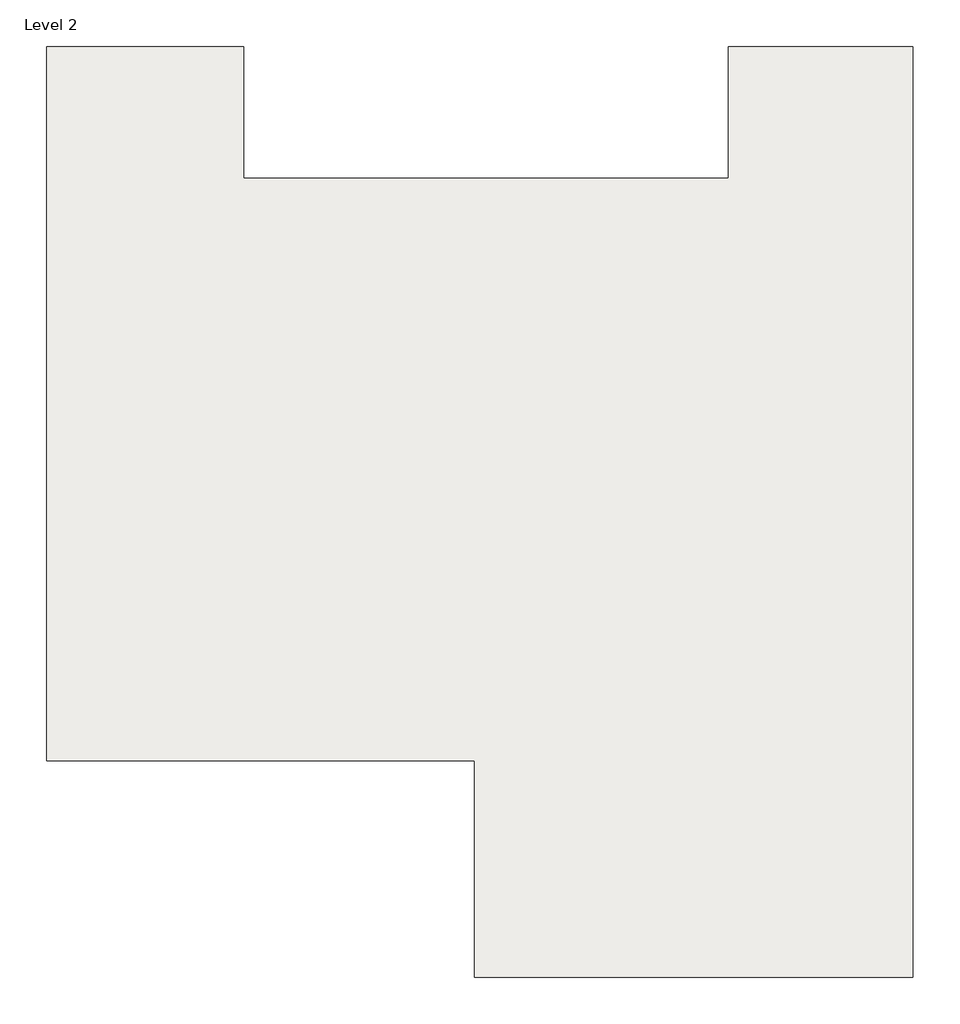
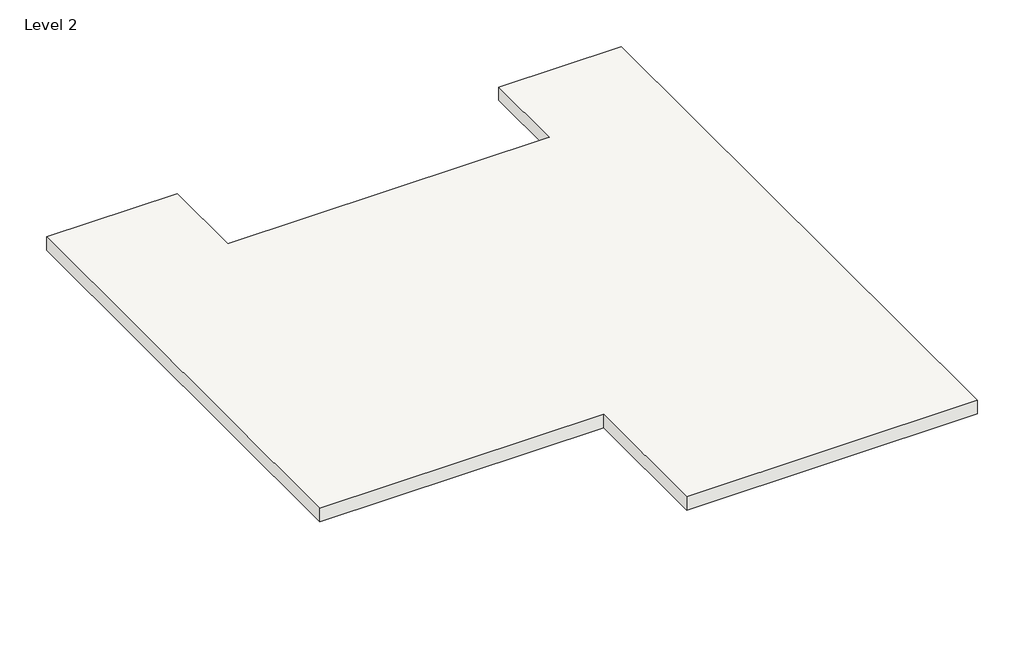
# One storey: 1 roof.
"""IFC4 building model written with IfcOpenShell, lengths in millimetres."""

from ifc_helpers import new_model, si_unit, frame, origin, place, context, project, spatial, polyline, outline, extrude, element, save

model = new_model("IFC4")

# Units and contexts
model_context = context("Model", 3, world=origin())
ifc_project = project(units=[si_unit("LENGTHUNIT", "METRE", prefix="MILLI")], contexts=[model_context])

# Site, building, storey
site = spatial("IfcSite", under=ifc_project)
building = spatial("IfcBuilding", under=site)
storey = spatial("IfcBuildingStorey", under=building, Name="Level 2", Elevation=3048.0)

# Roof
placement = place(None, origin())
element("IfcRoof", 1, ObjectType="Generic - 12\"", at=placement, inside=storey, context=model_context, shape_type="SweptSolid", body=[
    extrude(outline(polyline([(-392.7238552, 14768.0234128), (-392.7238552, 1547.3234128), (-392.7238552, 1458.4234128), (-6666.5238552, 1458.4234128), (-6666.5238552, 4557.2234128), (-12787.9238552, 4557.2234128), (-12787.9238552, 14768.0234128), (-9968.5238552, 14768.0234128), (-9968.5238552, 12888.4234128), (-3034.3238552, 12888.4234128), (-3034.3238552, 14768.0234128), (-392.7238552, 14768.0234128)])), frame((0.0, 0.0, 3048.0), z_axis=(0.0, 0.0, 1.0), x_axis=(1.0, 0.0, 0.0)), (0.0, 0.0, 1.0), 304.8),
])

save(model, "model.ifc")

# Revit data of these elements
# Type "Generic - 12\""
#   Assembly Code = "B1020"
#   Layers, outside or top first: 1' - 0" "Brick, Soldier Course" (function 1)
# Element 1 (IfcRoof, "Generic - 12\"")
#   built-in parameter 1001705 = 11 (stored number, unit not read)
#   built-in parameter 1001710 = 33615
#   Phase Created = New Construction
#   Materials on its faces: "Brick, Soldier Course"
# Materials
#   "Brick, Soldier Course": class "Masonry", colour RGB 170 98 104, transparency 0, Description = "Common brick soldier coursed", Cost = 0
